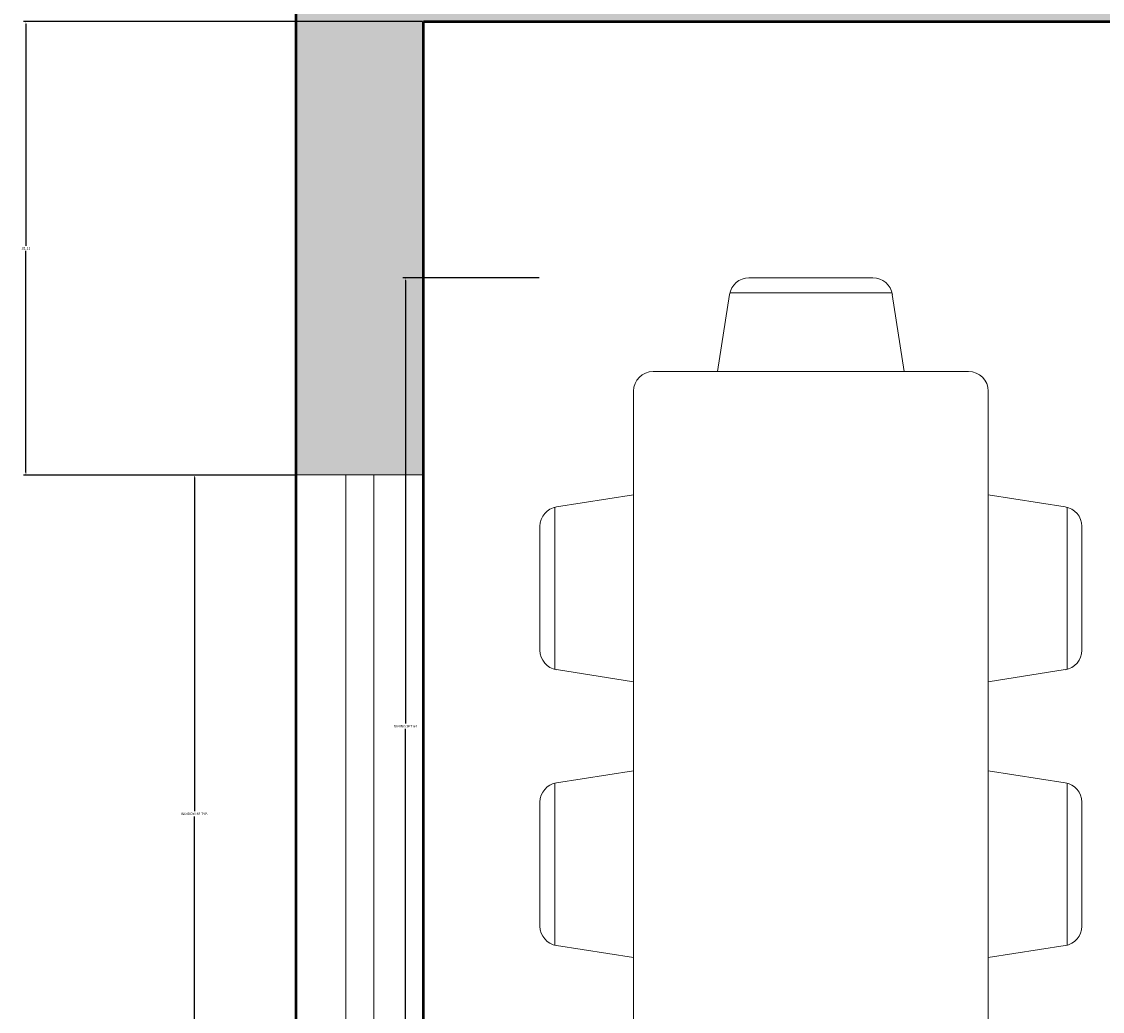
# Model space of a CAD drawing. Units: inches. Extents: x 2307 to 2544, y 2171 to 2540.
# Tile 15 of 52: x 2307 to 2384, y 2317 to 2388. Entities that reach past the tile are written whole.
import ezdxf

# ---------------------------------------------------------------- set-up
doc = ezdxf.new("R2010")
doc.units = ezdxf.units.IN
for name, color, linetype, lineweight in [('A-ANNO-DIMS', 2, 'Continuous', 18), ('A-FURN', 8, 'Continuous', 18), ('A-GLAZ', 4, 'Continuous', 18), ('A-WALL', 7, 'Continuous', 50)]:
    doc.layers.add(name, color=color, linetype=linetype, lineweight=lineweight)
doc.layers.add('A-WALL-PATT', color=18, linetype='Continuous', lineweight=13, true_color=0x000000)
doc.styles.get("Standard").update_dxf_attribs({"font": 'arial.ttf'})
doc.dimstyles.get("Standard").update_dxf_attribs({"dimtxt": 0.18, "dimasz": 0.18, "dimexe": 0.18, "dimexo": 0.0625, "dimgap": 0.09, "dimtad": 0, "dimtih": 1, "dimtoh": 1, "dimdec": 4, "dimzin": 0, "dimdsep": 46, "dimtxsty": 'Standard', "dimcen": 0.09, "dimadec": 0, "dimazin": 0, "dimtfac": 1, "dimtdec": 4, "dimtofl": 0, "dimtmove": 0, "dimatfit": 3, "dimfxl": 1, "dimtolj": 1, "dimtzin": 0, "dimarcsym": 0})

# ---------------------------------------------------------------- blocks, each defined once
blk = doc.blocks.new('Dining Set - 36 x 72 in.')
for p, q in [((-20.29, 27.5), (-7.71, 27.5)), ((7.71, 27.5), (20.29, 27.5)), ((-22.26, 25.81), (-23.48, 18)), ((-22.23, 26), (-5.76, 26)), ((-4.52, 18), (-5.74, 25.81)), ((5.74, 25.81), (4.52, 18)), ((5.77, 26), (22.24, 26)), ((23.48, 18), (22.26, 25.81)), ((34, 18), (-34, 18)), ((-36, 16), (-36, -16)), ((36, -16), (36, 16)), ((-43.81, 8.26), (-36, 9.48)), ((43.81, 8.26), (36, 9.48)), ((-44, 8.23), (-44, -8.24)), ((44, 8.23), (44, -8.24)), ((-45.5, 6.29), (-45.5, -6.29)), ((45.5, 6.29), (45.5, -6.29)), ((-36, -9.48), (-43.81, -8.26)), ((36, -9.48), (43.81, -8.26)), ((-34, -18), (34, -18)), ((-22.26, -25.81), (-23.48, -18)), ((-4.52, -18), (-5.74, -25.81)), ((5.74, -25.81), (4.52, -18)), ((23.48, -18), (22.26, -25.81)), ((-22.23, -26), (-5.76, -26)), ((5.77, -26), (22.24, -26)), ((-20.29, -27.5), (-7.71, -27.5)), ((7.71, -27.5), (20.29, -27.5))]:
    blk.add_line(p, q)
for centre, start, end in [((-20.29, 25.5), 90, 171.1198), ((-7.71, 25.5), 8.881, 90), ((7.71, 25.5), 90, 171.1198), ((20.29, 25.5), 8.881, 90), ((-34, 16), 90, 180), ((34, 16), 0, 90), ((-43.5, 6.29), 98.8806, 180), ((43.5, 6.29), 0, 81.1194), ((-43.5, -6.29), 180, 261.1194), ((43.5, -6.29), 278.8806, 0), ((-34, -16), 180, 270), ((34, -16), 270, 0), ((-20.29, -25.5), 188.8802, 270), ((-7.71, -25.5), 270, 351.1191), ((7.71, -25.5), 188.8802, 270), ((20.29, -25.5), 270, 351.1191)]:
    blk.add_arc(centre, 2, start, end)
blk = doc.blocks.new('WIN-48IN')
for p, q in [((0, 5.5), (48, 5.5)), ((0, 3.5), (48, 3.5))]:
    blk.add_line(p, q)
for points in [[(0, 0), (0, 9)], [(48, 9), (48, 0)]]:
    blk.add_lwpolyline(points)
blk = doc.blocks.new('*D16')
at = {"layer": 'A-ANNO-DIMS', "color": 0, "lineweight": -2, "transparency": 16777216}
for p, q in [((2326.633, 2355.398), (2319.316, 2355.398)), ((2319.496, 2355.218), (2319.496, 2331.581)), ((2319.496, 2307.578), (2319.496, 2331.215)), ((2326.633, 2307.398), (2319.316, 2307.398))]:
    blk.add_line(p, q, dxfattribs=at)
at = {"layer": 'A-ANNO-DIMS', "color": 0, "transparency": 16777216}
for points in [[(2319.466, 2355.218), (2319.526, 2355.218), (2319.496, 2355.398)], [(2319.466, 2307.578), (2319.526, 2307.578), (2319.496, 2307.398)]]:
    blk.add_solid(points, dxfattribs=at)
at = {"layer": 'Defpoints', "color": 0, "transparency": 16777216}
for p in [(2326.696, 2355.398), (2319.496, 2307.398), (2326.696, 2307.398)]:
    blk.add_point(p, dxfattribs=at)
at = {"layer": 'A-ANNO-DIMS', "color": 0, "transparency": 16777216, "insert": (2319.496, 2331.398), "char_height": 0.18, "attachment_point": 5}
blk.add_mtext('\\A1;WINDOW 48 TYP.', dxfattribs=at)
blk = doc.blocks.new('*D28')
at = {"layer": 'A-ANNO-DIMS', "color": 0, "lineweight": -2, "transparency": 16777216}
for p, q in [((2343.895, 2369.359), (2334.252, 2369.359)), ((2334.432, 2369.179), (2334.432, 2337.789)), ((2334.432, 2306.032), (2334.432, 2337.423)), ((2343.895, 2305.852), (2334.252, 2305.852))]:
    blk.add_line(p, q, dxfattribs=at)
at = {"layer": 'A-ANNO-DIMS', "color": 0, "transparency": 16777216}
for points in [[(2334.402, 2369.179), (2334.462, 2369.179), (2334.432, 2369.359)], [(2334.402, 2306.032), (2334.462, 2306.032), (2334.432, 2305.852)]]:
    blk.add_solid(points, dxfattribs=at)
at = {"layer": 'Defpoints', "color": 0, "transparency": 16777216}
for p in [(2343.958, 2369.359), (2334.432, 2305.852), (2343.958, 2305.852)]:
    blk.add_point(p, dxfattribs=at)
at = {"layer": 'A-ANNO-DIMS', "color": 0, "transparency": 16777216, "insert": (2334.432, 2337.606), "char_height": 0.18, "attachment_point": 5}
blk.add_mtext('\\A1;DINING SET 64', dxfattribs=at)
blk = doc.blocks.new('*D41')
at = {"layer": 'A-ANNO-DIMS', "color": 0, "lineweight": -2, "transparency": 16777216}
for p, q in [((2335.633, 2387.51), (2307.366, 2387.51)), ((2307.546, 2387.33), (2307.546, 2371.636)), ((2307.546, 2355.578), (2307.546, 2371.272)), ((2326.633, 2355.398), (2307.366, 2355.398))]:
    blk.add_line(p, q, dxfattribs=at)
at = {"layer": 'A-ANNO-DIMS', "color": 0, "transparency": 16777216}
for points in [[(2307.516, 2387.33), (2307.576, 2387.33), (2307.546, 2387.51)], [(2307.516, 2355.578), (2307.576, 2355.578), (2307.546, 2355.398)]]:
    blk.add_solid(points, dxfattribs=at)
at = {"layer": 'Defpoints', "color": 0, "transparency": 16777216}
for p in [(2307.546, 2387.51), (2335.696, 2387.51), (2326.696, 2355.398)]:
    blk.add_point(p, dxfattribs=at)
at = {"layer": 'A-ANNO-DIMS', "color": 0, "transparency": 16777216, "insert": (2307.546, 2371.454), "char_height": 0.18, "attachment_point": 5}
blk.add_mtext('\\A1;32.11', dxfattribs=at)

msp = doc.modelspace()

# ---------------------------------------------------------------- hatches: boundary and pattern name
at = {"layer": 'A-WALL-PATT'}
h = msp.add_hatch(color=256, dxfattribs=at)
h.dxf.hatch_style = 1
h.paths.add_polyline_path([(2367.4028, 2520.5096), (2326.6958, 2520.5096), (2326.6958, 2355.3983), (2335.6958, 2355.3983), (2335.6958, 2387.5096), (2415.6958, 2387.5096), (2415.6958, 2391.5096), (2335.6958, 2391.5096), (2335.6958, 2409.5096), (2335.6958, 2511.5096), (2367.4028, 2511.5096)])

# ---------------------------------------------------------------- linework, layer by layer
at = {"layer": 'A-WALL'}
for p, q in [((2335.6958, 2199.5096), (2335.6958, 2387.5096)), ((2335.6958, 2387.5096), (2415.6958, 2387.5096))]:
    msp.add_line(p, q, dxfattribs=at)
msp.add_lwpolyline([(2433.7832, 2190.5096), (2326.6958, 2190.5096), (2326.6958, 2520.5096), (2524.6958, 2520.5096), (2524.6958, 2190.5096), (2469.785, 2190.5096)], dxfattribs=at)

# ---------------------------------------------------------------- block references
at = {"layer": 'A-FURN', "xscale": 0.697875586402136, "yscale": 0.697875586402136, "zscale": 0.697875586402136, "rotation": 270}
msp.add_blockref('Dining Set - 36 x 72 in.', (2363.1494, 2337.6056), dxfattribs=at)
at = {"layer": 'A-GLAZ', "rotation": 270.0000000000004}
msp.add_blockref('WIN-48IN', (2326.6963, 2355.3986), dxfattribs=at)

# ---------------------------------------------------------------- dimensions: what is measured, and where the dimension line sits
at = {"layer": 'A-ANNO-DIMS'}
dim = msp.add_linear_dim(base=(2307.5458, 2387.5096), p1=(2326.6958, 2355.3983), p2=(2335.6958, 2387.5096), angle=90, dimstyle='Standard', override={"dimdec": 2, "dimlfac": 1, "dimrnd": 0, "dimzin": 0, "dimdsep": 46, "dimlunit": 2}, dxfattribs=at)
dim.commit()
dim.dimension.update_dxf_attribs({"geometry": '*D41', "text_midpoint": (2307.5458, 2371.4539)})
for base, p1, p2, text, picture, middle in [((2334.4318, 2305.8523), (2343.9578, 2369.3589), (2343.9578, 2305.8523), 'DINING SET <>', '*D28', (2334.4318, 2337.6056)), ((2319.4958, 2307.3983), (2326.6958, 2355.3983), (2326.6958, 2307.3983), 'WINDOW <> TYP.', '*D16', (2319.4958, 2331.3983))]:
    dim = msp.add_linear_dim(base=base, p1=p1, p2=p2, angle=270, text=text, dimstyle='Standard', override={"dimdec": 0, "dimlfac": 1, "dimrnd": 0, "dimzin": 0, "dimdsep": 46, "dimlunit": 2}, dxfattribs=at)
    dim.commit()
    dim.dimension.update_dxf_attribs({"geometry": picture, "text_midpoint": middle})

doc.saveas('drawing.dxf')
